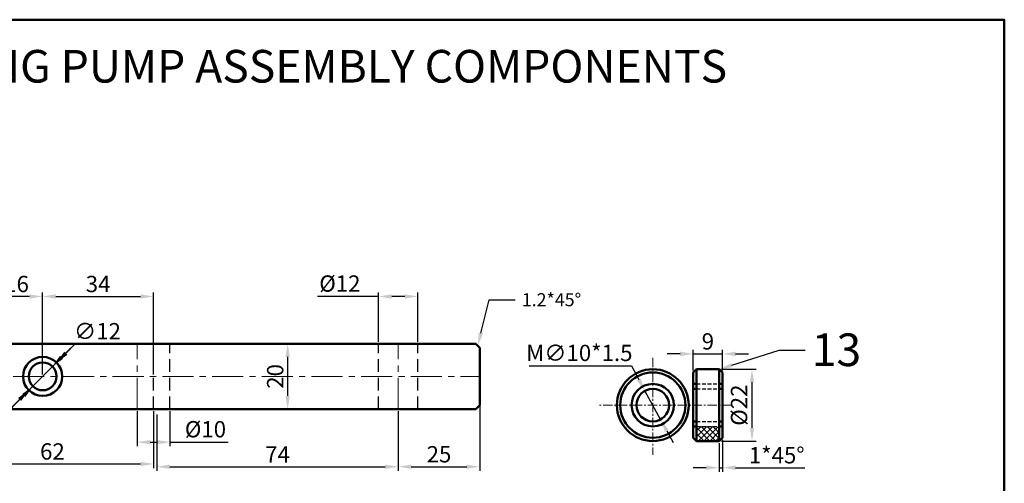
# Model space of a CAD drawing. Units: millimetres. Extents: x 24 to 508, y -182 to 223.
# Tile 6 of 6: x 207 to 508, y 81 to 223. Entities that reach past the tile are written whole.
import ezdxf
from ezdxf import colors
from ezdxf.entities.mleader import LeaderData, LeaderLine
from ezdxf.math import Vec2, Vec3

# ---------------------------------------------------------------- set-up
doc = ezdxf.new("R2010")
doc.units = ezdxf.units.MM
doc.header["$LTSCALE"] = 0.3
doc.linetypes.add('CENTER', pattern=[50.8, 31.75, -6.35, 6.35, -6.35])
doc.linetypes.add('DASHED', pattern=[19.05, 12.7, -6.35])
for name, color, linetype, lineweight in [('M-CNTR', 1, 'CENTER', 18), ('M-DIMS', 2, 'Continuous', 25), ('M-HATC', 8, 'Continuous', 18), ('M-HIDN', 4, 'DASHED', 25), ('M-OUTL', 7, 'Continuous', 50), ('M-TEXT', 7, 'Continuous', 25)]:
    doc.layers.add(name, color=color, linetype=linetype, lineweight=lineweight)
doc.styles.get("Standard").update_dxf_attribs({"font": 'arial.ttf'})
doc.dimstyles.new('ISO-25', dxfattribs={"dimtxt": 5, "dimasz": 4, "dimexe": 1.25, "dimexo": 0.625, "dimtad": 1, "dimtoh": 1, "dimdec": 0, "dimtxsty": 'Standard', "dimcen": 2.5, "dimadec": 0, "dimazin": 0, "dimtfac": 1, "dimtdec": 0, "dimtmove": 0, "dimatfit": 3, "dimfxl": 1, "dimarcsym": 0})

# ---------------------------------------------------------------- blocks, each defined once
blk = doc.blocks.new('*D8')
at = {"layer": 'Defpoints', "color": 0, "ltscale": 0.3, "transparency": 16777216}
for p in [(197.61, 137.94), (197.61, 113.44), (213.61, 113.44)]:
    blk.add_point(p, dxfattribs=at)
at = {"layer": 'M-DIMS', "color": 0, "lineweight": -2, "ltscale": 0.3, "transparency": 16777216}
for p, q in [((197.61, 114.07), (197.61, 139.19)), ((213.61, 114.07), (213.61, 139.19)), ((209.61, 137.94), (201.61, 137.94))]:
    blk.add_line(p, q, dxfattribs=at)
at = {"layer": 'M-DIMS', "color": 0, "ltscale": 0.3, "transparency": 16777216}
for points in [[(201.61, 138.6), (201.61, 137.27), (197.61, 137.94)], [(209.61, 138.6), (209.61, 137.27), (213.61, 137.94)]]:
    blk.add_solid(points, dxfattribs=at)
at = {"layer": 'M-DIMS', "color": 0, "ltscale": 0.3, "transparency": 16777216, "insert": (205.61, 141.11), "char_height": 5, "attachment_point": 5}
blk.add_mtext('16', dxfattribs=at)
blk = doc.blocks.new('*D9')
at = {"layer": 'Defpoints', "color": 0, "ltscale": 0.3, "transparency": 16777216}
for p in [(247.61, 137.94), (213.61, 113.44), (247.61, 113.44)]:
    blk.add_point(p, dxfattribs=at)
at = {"layer": 'M-DIMS', "color": 0, "lineweight": -2, "ltscale": 0.3, "transparency": 16777216}
for p, q in [((213.61, 114.07), (213.61, 139.19)), ((247.61, 114.07), (247.61, 139.19)), ((217.61, 137.94), (243.61, 137.94))]:
    blk.add_line(p, q, dxfattribs=at)
at = {"layer": 'M-DIMS', "color": 0, "ltscale": 0.3, "transparency": 16777216}
for points in [[(217.61, 138.6), (217.61, 137.27), (213.61, 137.94)], [(243.61, 138.6), (243.61, 137.27), (247.61, 137.94)]]:
    blk.add_solid(points, dxfattribs=at)
at = {"layer": 'M-DIMS', "color": 0, "ltscale": 0.3, "transparency": 16777216, "insert": (230.61, 141.12), "char_height": 5, "attachment_point": 5}
blk.add_mtext('34', dxfattribs=at)
blk = doc.blocks.new('*D10')
at = {"layer": 'Defpoints', "color": 0, "ltscale": 0.3, "transparency": 16777216}
for p in [(242.61, 103.44), (252.61, 103.44), (252.61, 93.29)]:
    blk.add_point(p, dxfattribs=at)
at = {"layer": 'M-DIMS', "color": 0, "lineweight": -2, "ltscale": 0.3, "transparency": 16777216}
for p, q in [((242.61, 102.82), (242.61, 92.04)), ((252.61, 102.82), (252.61, 92.04)), ((246.61, 93.29), (248.61, 93.29)), ((252.61, 93.29), (270.44, 93.29))]:
    blk.add_line(p, q, dxfattribs=at)
at = {"layer": 'M-DIMS', "color": 0, "ltscale": 0.3, "transparency": 16777216}
for points in [[(246.61, 93.96), (246.61, 92.63), (242.61, 93.29)], [(248.61, 93.96), (248.61, 92.63), (252.61, 93.29)]]:
    blk.add_solid(points, dxfattribs=at)
at = {"layer": 'M-DIMS', "color": 0, "ltscale": 0.3, "transparency": 16777216, "insert": (263.52, 96.61), "char_height": 5, "attachment_point": 5}
blk.add_mtext('%%C10', dxfattribs=at)
blk = doc.blocks.new('*D11')
at = {"layer": 'Defpoints', "color": 0, "ltscale": 0.3, "transparency": 16777216}
for p in [(290.14, 123.44), (288.72, 103.44), (290.14, 103.44)]:
    blk.add_point(p, dxfattribs=at)
at = {"layer": 'M-DIMS', "color": 0, "lineweight": -2, "ltscale": 0.3, "transparency": 16777216}
for p, q in [((289.51, 123.44), (287.47, 123.44)), ((288.72, 119.44), (288.72, 107.44)), ((289.51, 103.44), (287.47, 103.44))]:
    blk.add_line(p, q, dxfattribs=at)
at = {"layer": 'M-DIMS', "color": 0, "ltscale": 0.3, "transparency": 16777216}
for points in [[(288.05, 119.44), (289.39, 119.44), (288.72, 123.44)], [(288.05, 107.44), (289.39, 107.44), (288.72, 103.44)]]:
    blk.add_solid(points, dxfattribs=at)
at = {"layer": 'M-DIMS', "color": 0, "ltscale": 0.3, "transparency": 16777216, "insert": (285.54, 113.44), "char_height": 5, "attachment_point": 5, "rotation": 90}
blk.add_mtext('20', dxfattribs=at)
blk = doc.blocks.new('*D12')
at = {"layer": 'Defpoints', "color": 0, "ltscale": 0.3, "transparency": 16777216}
for p in [(347.61, 113.44), (322.61, 103.44), (347.61, 85.77)]:
    blk.add_point(p, dxfattribs=at)
at = {"layer": 'M-DIMS', "color": 0, "lineweight": -2, "ltscale": 0.3, "transparency": 16777216}
for p, q in [((347.61, 112.82), (347.61, 84.52)), ((322.61, 102.82), (322.61, 84.52)), ((326.61, 85.77), (343.61, 85.77))]:
    blk.add_line(p, q, dxfattribs=at)
at = {"layer": 'M-DIMS', "color": 0, "ltscale": 0.3, "transparency": 16777216}
for points in [[(326.61, 86.43), (326.61, 85.1), (322.61, 85.77)], [(343.61, 86.43), (343.61, 85.1), (347.61, 85.77)]]:
    blk.add_solid(points, dxfattribs=at)
at = {"layer": 'M-DIMS', "color": 0, "ltscale": 0.3, "transparency": 16777216, "insert": (335.11, 88.94), "char_height": 5, "attachment_point": 5}
blk.add_mtext('25', dxfattribs=at)
blk = doc.blocks.new('*D13')
at = {"layer": 'Defpoints', "color": 0, "ltscale": 0.3, "transparency": 16777216}
for p in [(247.61, 103.44), (185.61, 97.23), (247.61, 86.62)]:
    blk.add_point(p, dxfattribs=at)
at = {"layer": 'M-DIMS', "color": 0, "lineweight": -2, "ltscale": 0.3, "transparency": 16777216}
for p, q in [((247.61, 102.82), (247.61, 85.37)), ((185.61, 96.6), (185.61, 85.37)), ((189.61, 86.62), (243.61, 86.62))]:
    blk.add_line(p, q, dxfattribs=at)
at = {"layer": 'M-DIMS', "color": 0, "ltscale": 0.3, "transparency": 16777216}
for points in [[(189.61, 87.28), (189.61, 85.95), (185.61, 86.62)], [(243.61, 87.28), (243.61, 85.95), (247.61, 86.62)]]:
    blk.add_solid(points, dxfattribs=at)
at = {"layer": 'M-DIMS', "color": 0, "ltscale": 0.3, "transparency": 16777216, "insert": (216.61, 89.8), "char_height": 5, "attachment_point": 5}
blk.add_mtext('62', dxfattribs=at)
blk = doc.blocks.new('*D14')
at = {"layer": 'Defpoints', "color": 0, "ltscale": 0.3, "transparency": 16777216}
for p in [(322.61, 103.44), (248.61, 102.44), (322.61, 85.77)]:
    blk.add_point(p, dxfattribs=at)
at = {"layer": 'M-DIMS', "color": 0, "lineweight": -2, "ltscale": 0.3, "transparency": 16777216}
for p, q in [((322.61, 102.82), (322.61, 84.52)), ((248.61, 101.82), (248.61, 84.52)), ((252.61, 85.77), (318.61, 85.77))]:
    blk.add_line(p, q, dxfattribs=at)
at = {"layer": 'M-DIMS', "color": 0, "ltscale": 0.3, "transparency": 16777216}
for points in [[(252.61, 86.43), (252.61, 85.1), (248.61, 85.77)], [(318.61, 86.43), (318.61, 85.1), (322.61, 85.77)]]:
    blk.add_solid(points, dxfattribs=at)
at = {"layer": 'M-DIMS', "color": 0, "ltscale": 0.3, "transparency": 16777216, "insert": (285.61, 88.89), "char_height": 5, "attachment_point": 5}
blk.add_mtext('74', dxfattribs=at)
blk = doc.blocks.new('*D15')
at = {"layer": 'Defpoints', "color": 0, "ltscale": 0.3, "transparency": 16777216}
for p in [(328.61, 137.94), (316.61, 123.44), (328.61, 123.44)]:
    blk.add_point(p, dxfattribs=at)
at = {"layer": 'M-DIMS', "color": 0, "lineweight": -2, "ltscale": 0.3, "transparency": 16777216}
for p, q in [((316.61, 124.07), (316.61, 139.19)), ((328.61, 124.07), (328.61, 139.19)), ((316.61, 137.94), (297.83, 137.94)), ((324.61, 137.94), (320.61, 137.94))]:
    blk.add_line(p, q, dxfattribs=at)
at = {"layer": 'M-DIMS', "color": 0, "ltscale": 0.3, "transparency": 16777216}
for points in [[(320.61, 138.6), (320.61, 137.27), (316.61, 137.94)], [(324.61, 138.6), (324.61, 137.27), (328.61, 137.94)]]:
    blk.add_solid(points, dxfattribs=at)
at = {"layer": 'M-DIMS', "color": 0, "ltscale": 0.3, "transparency": 16777216, "insert": (304.73, 141.25), "char_height": 5, "attachment_point": 5}
blk.add_mtext('%%C12', dxfattribs=at)
blk = doc.blocks.new('*D26')
at = {"layer": 'Defpoints', "color": 0, "ltscale": 0.3, "transparency": 16777216}
for p in [(398.26, 109.03), (403.06, 100.25)]:
    blk.add_point(p, dxfattribs=at)
at = {"layer": 'M-DIMS', "color": 0, "lineweight": -2, "ltscale": 0.3, "transparency": 16777216}
for p, q in [((362.81, 116.67), (394.09, 116.67)), ((394.09, 116.67), (396.35, 112.54)), ((403.06, 100.25), (398.26, 109.03)), ((404.97, 96.74), (406.89, 93.23))]:
    blk.add_line(p, q, dxfattribs=at)
at = {"layer": 'M-DIMS', "color": 0, "ltscale": 0.3, "transparency": 16777216}
for points in [[(396.93, 112.86), (395.76, 112.22), (398.26, 109.03)], [(405.56, 97.06), (404.39, 96.42), (403.06, 100.25)]]:
    blk.add_solid(points, dxfattribs=at)
at = {"layer": 'M-DIMS', "color": 0, "ltscale": 0.3, "transparency": 16777216, "insert": (378.14, 119.99), "char_height": 5, "attachment_point": 5}
blk.add_mtext('M∅10*1.5', dxfattribs=at)
blk = doc.blocks.new('*D27')
at = {"layer": 'Defpoints', "color": 0, "ltscale": 0.3, "transparency": 16777216}
for p in [(421.05, 115.64), (421.05, 93.64), (431.07, 93.64)]:
    blk.add_point(p, dxfattribs=at)
at = {"layer": 'M-DIMS', "color": 0, "lineweight": -2, "ltscale": 0.3, "transparency": 16777216}
for p, q in [((421.68, 115.64), (432.32, 115.64)), ((431.07, 111.64), (431.07, 97.64)), ((421.68, 93.64), (432.32, 93.64))]:
    blk.add_line(p, q, dxfattribs=at)
at = {"layer": 'M-DIMS', "color": 0, "ltscale": 0.3, "transparency": 16777216}
for points in [[(430.41, 111.64), (431.74, 111.64), (431.07, 115.64)], [(430.41, 97.64), (431.74, 97.64), (431.07, 93.64)]]:
    blk.add_solid(points, dxfattribs=at)
at = {"layer": 'M-DIMS', "color": 0, "ltscale": 0.3, "transparency": 16777216, "insert": (427.76, 104.64), "char_height": 5, "attachment_point": 5, "rotation": 90}
blk.add_mtext('%%C22', dxfattribs=at)
blk = doc.blocks.new('*D28')
at = {"layer": 'Defpoints', "color": 0, "ltscale": 0.3, "transparency": 16777216}
for p in [(422.05, 120.34), (413.05, 114.64), (422.05, 114.64)]:
    blk.add_point(p, dxfattribs=at)
at = {"layer": 'M-DIMS', "color": 0, "lineweight": -2, "ltscale": 0.3, "transparency": 16777216}
for p, q in [((413.05, 115.27), (413.05, 121.59)), ((422.05, 115.27), (422.05, 121.59)), ((409.05, 120.34), (405.05, 120.34)), ((413.05, 120.34), (422.05, 120.34)), ((426.05, 120.34), (430.05, 120.34))]:
    blk.add_line(p, q, dxfattribs=at)
at = {"layer": 'M-DIMS', "color": 0, "ltscale": 0.3, "transparency": 16777216}
for points in [[(409.05, 121.01), (409.05, 119.67), (413.05, 120.34)], [(426.05, 121.01), (426.05, 119.67), (422.05, 120.34)]]:
    blk.add_solid(points, dxfattribs=at)
at = {"layer": 'M-DIMS', "color": 0, "ltscale": 0.3, "transparency": 16777216, "insert": (417.55, 123.52), "char_height": 5, "attachment_point": 5}
blk.add_mtext('9', dxfattribs=at)
blk = doc.blocks.new('*D29')
at = {"layer": 'Defpoints', "color": 0, "ltscale": 0.3, "transparency": 16777216}
for p in [(421.05, 93.64), (422.05, 94.64), (422.05, 85.46)]:
    blk.add_point(p, dxfattribs=at)
at = {"layer": 'M-DIMS', "color": 0, "lineweight": -2, "ltscale": 0.3, "transparency": 16777216}
for p, q in [((422.05, 94.02), (422.05, 84.21)), ((421.05, 93.02), (421.05, 84.21)), ((417.05, 85.46), (413.05, 85.46)), ((421.05, 85.46), (422.05, 85.46)), ((426.05, 85.46), (447.24, 85.46))]:
    blk.add_line(p, q, dxfattribs=at)
at = {"layer": 'M-DIMS', "color": 0, "ltscale": 0.3, "transparency": 16777216}
for points in [[(417.05, 86.13), (417.05, 84.8), (421.05, 85.46)], [(426.05, 86.13), (426.05, 84.8), (422.05, 85.46)]]:
    blk.add_solid(points, dxfattribs=at)
at = {"layer": 'M-DIMS', "color": 0, "ltscale": 0.3, "transparency": 16777216, "insert": (438.65, 88.64), "char_height": 5, "attachment_point": 5}
blk.add_mtext('1*45%%D', dxfattribs=at)
blk = doc.blocks.new('*D79')
at = {"layer": 'Defpoints', "color": 0, "ltscale": 0.3, "transparency": 16777216}
for p in [(217.85, 117.68), (209.36, 109.2)]:
    blk.add_point(p, dxfattribs=at)
at = {"layer": 'M-DIMS', "color": 0, "lineweight": -2, "ltscale": 0.3, "transparency": 16777216}
for p, q in [((223.51, 123.34), (220.68, 120.51)), ((236.69, 123.34), (223.51, 123.34)), ((209.36, 109.2), (217.85, 117.68)), ((206.53, 106.37), (203.7, 103.55))]:
    blk.add_line(p, q, dxfattribs=at)
at = {"layer": 'M-DIMS', "color": 0, "ltscale": 0.3, "transparency": 16777216}
for points in [[(220.21, 120.98), (221.15, 120.04), (217.85, 117.68)], [(206.06, 106.84), (207, 105.9), (209.36, 109.2)]]:
    blk.add_solid(points, dxfattribs=at)
at = {"layer": 'M-DIMS', "color": 0, "ltscale": 0.3, "transparency": 16777216, "insert": (230.41, 126.65), "char_height": 5, "attachment_point": 5}
blk.add_mtext('∅12', dxfattribs=at)
blk = doc.blocks.new('*D80')
at = {"layer": 'Defpoints', "color": 0, "ltscale": 0.3, "transparency": 16777216}
for p in [(216.59, 116.46), (210.62, 110.42)]:
    blk.add_point(p, dxfattribs=at)
at = {"layer": 'M-DIMS', "color": 0, "lineweight": -2, "ltscale": 0.3, "transparency": 16777216}
for p, q in [((219.41, 119.31), (222.22, 122.15)), ((216.59, 116.46), (210.62, 110.42)), ((201.21, 100.9), (207.81, 107.57)), ((186, 100.9), (201.21, 100.9))]:
    blk.add_line(p, q, dxfattribs=at)
at = {"layer": 'M-DIMS', "color": 0, "ltscale": 0.3, "transparency": 16777216}
for points in [[(218.93, 119.78), (219.88, 118.84), (216.59, 116.46)], [(207.33, 108.04), (208.28, 107.11), (210.62, 110.42)]]:
    blk.add_solid(points, dxfattribs=at)
at = {"layer": 'M-DIMS', "color": 0, "ltscale": 0.3, "transparency": 16777216, "insert": (193.29, 104.22), "char_height": 5, "attachment_point": 5}
blk.add_mtext('∅8.5', dxfattribs=at)

msp = doc.modelspace()

# ---------------------------------------------------------------- hatches: boundary and pattern name
at = {"layer": 'M-HATC', "ltscale": 0.3}
h = msp.add_hatch(dxfattribs=at)
h.set_pattern_fill('ANSI37', color=256, scale=0.4)
h.set_pattern_definition([(45, (7.7601, 76.6072), (-0.8980256, 0.8980256), []), (135, (7.7601, 76.6072), (-0.8980256, -0.8980256), [])])
h.paths.add_polyline_path([(414.0501, 98.1407), (414.0501, 93.6407), (421.0501, 93.6407), (421.0501, 98.1407)])

# ---------------------------------------------------------------- linework, layer by layer
at = {"layer": 'M-CNTR'}
for p, q in [((242.6065, 103.4403), (242.6065, 123.4403)), ((322.6065, 103.4403), (322.6065, 123.4403)), ((82.668, 113.4403), (347.6065, 113.4403))]:
    msp.add_line(p, q, dxfattribs=at)
at = {"layer": 'M-CNTR', "ltscale": 0.3}
for p, q in [((400.6605, 119.1069), (400.6605, 89.3694)), ((424.8527, 104.6407), (384.1108, 104.6407))]:
    msp.add_line(p, q, dxfattribs=at)
at = {"layer": 'M-HIDN'}
for p, q in [((247.6065, 103.4403), (247.6065, 123.4403)), ((252.6065, 103.4403), (252.6065, 123.4403)), ((316.6065, 103.4403), (316.6065, 123.4403)), ((328.6065, 103.4403), (328.6065, 123.4403))]:
    msp.add_line(p, q, dxfattribs=at)
at = {"layer": 'M-HIDN', "ltscale": 0.3}
for p, q in [((414.0501, 111.1407), (421.0501, 111.1407)), ((414.0501, 109.6407), (421.0501, 109.6407)), ((414.0501, 99.6407), (421.0501, 99.6407)), ((414.0501, 98.1407), (421.0501, 98.1407))]:
    msp.add_line(p, q, dxfattribs=at)
at = {"layer": 'M-OUTL'}
for p, q in [((346.4065, 123.4403), (199.6065, 123.4403)), ((346.4065, 123.4403), (347.6065, 122.2403)), ((347.6065, 104.6403), (347.6065, 122.2403)), ((346.4065, 103.4403), (199.6065, 103.4403)), ((347.6065, 104.6403), (346.4065, 103.4403))]:
    msp.add_line(p, q, dxfattribs=at)
at = {"layer": 'M-OUTL', "ltscale": 0.3}
for p, q in [((413.0501, 114.6407), (414.0501, 115.6407)), ((414.0501, 115.6407), (421.0501, 115.6407)), ((414.0501, 93.6407), (414.0501, 115.6407)), ((421.0501, 115.6407), (421.0501, 93.6407)), ((422.0501, 114.6407), (421.0501, 115.6407)), ((413.0501, 94.6407), (413.0501, 114.6407)), ((422.0501, 114.6407), (422.0501, 94.6407)), ((414.0501, 111.1407), (413.0501, 111.1407)), ((414.0501, 109.6407), (413.0501, 109.6407)), ((421.0501, 111.1407), (422.0501, 111.1407)), ((421.0501, 109.6407), (422.0501, 109.6407)), ((414.0501, 99.6407), (413.0501, 99.6407)), ((421.0501, 99.6407), (422.0501, 99.6407)), ((414.0501, 98.1407), (413.0501, 98.1407)), ((421.0501, 98.1407), (422.0501, 98.1407)), ((413.0501, 94.6407), (414.0501, 93.6407)), ((421.0501, 93.6407), (414.0501, 93.6407)), ((422.0501, 94.6407), (421.0501, 93.6407))]:
    msp.add_line(p, q, dxfattribs=at)
msp.add_lwpolyline([(23.7253, 222.7463), (508.4225, 222.7463), (508.4225, -181.5799), (23.7253, -181.5799)], close=True, dxfattribs=at)
at = {"layer": 'M-OUTL'}
for radius in [6, 4.25]:
    msp.add_circle((213.6065, 113.4403), radius, dxfattribs=at)
at = {"layer": 'M-OUTL', "ltscale": 0.3}
for radius in [11, 10, 6.5, 5]:
    msp.add_circle((400.6605, 104.6407), radius, dxfattribs=at)

# ---------------------------------------------------------------- texts
at = {"layer": 'M-TEXT', "ltscale": 0.3, "insert": (130.5797, 213.4834), "char_height": 10, "attachment_point": 1}
msp.add_mtext_dynamic_manual_height_columns('OSCILLATING PUMP ASSEMBLY COMPONENTS', width=327.515557, gutter_width=12.5, heights=[0], dxfattribs=at)

# ---------------------------------------------------------------- dimensions: what is measured, and where the dimension line sits
at = {"layer": 'M-DIMS', "ltscale": 0.3}
for base, p1, p2, picture, middle in [((197.6065, 137.9361), (213.6065, 113.4403), (197.6065, 113.4403), '*D8', (205.6065, 141.114)), ((247.6065, 137.9361), (213.6065, 113.4403), (247.6065, 113.4403), '*D9', (230.6065, 141.1157)), ((422.0501, 120.339), (413.0501, 114.6407), (422.0501, 114.6407), '*D28', (417.5501, 123.5169)), ((347.6065, 85.7656), (322.6065, 103.4403), (347.6065, 113.4403), '*D12', (335.1065, 88.9435)), ((247.6065, 86.6173), (185.6065, 97.2279), (247.6065, 103.4403), '*D13', (216.6065, 89.7952)), ((322.6065, 85.7656), (248.6065, 102.4403), (322.6065, 103.4403), '*D14', (285.6065, 88.8906))]:
    dim = msp.add_linear_dim(base=base, p1=p1, p2=p2, dimstyle='ISO-25', override={"dimclrd": 0, "dimclre": 0, "dimclrt": 0}, dxfattribs=at)
    dim.commit()
    dim.dimension.update_dxf_attribs({"geometry": picture, "text_midpoint": middle})
for base, p1, p2, picture, middle in [((328.6065, 137.9361), (316.6065, 123.4403), (328.6065, 123.4403), '*D15', (304.7306, 137.9361)), ((252.6065, 93.2948), (242.6065, 103.4403), (252.6065, 103.4403), '*D10', (263.5241, 93.2948))]:
    dim = msp.add_linear_dim(base=base, p1=p1, p2=p2, text='%%C<>', dimstyle='ISO-25', override={"dimclrd": 0, "dimclre": 0, "dimclrt": 0}, dxfattribs=at)
    dim.commit()
    dim.dimension.update_dxf_attribs({"geometry": picture, "text_midpoint": middle, "dimtype": 160})
for p1, p2, override, picture, middle in [((209.3619, 109.1996), (217.8511, 117.6811), {"dimdec": 0, "dimlfac": 1, "dimrnd": 0, "dimzin": 0, "dimdsep": 46, "dimlunit": 2}, '*D79', (230.4111, 123.3353)), ((216.5948, 116.4623), (210.6182, 110.4184), {"dimdec": 1, "dimlfac": 1, "dimrnd": 0, "dimzin": 0, "dimdsep": 46, "dimlunit": 2}, '*D80', (193.2911, 100.9006))]:
    dim = msp.add_diameter_dim_2p(p1=p1, p2=p2, dimstyle='ISO-25', override=override, dxfattribs=at)
    dim.commit()
    dim.dimension.update_dxf_attribs({"geometry": picture, "text_midpoint": middle, "dimtype": 163})
dim = msp.add_linear_dim(base=(288.7205, 103.4403), p1=(290.1379, 123.4403), p2=(290.1379, 103.4403), angle=90, dimstyle='ISO-25', override={"dimclrd": 0, "dimclre": 0, "dimclrt": 0}, dxfattribs=at)
dim.commit()
dim.dimension.update_dxf_attribs({"geometry": '*D11', "text_midpoint": (285.5426, 113.4403)})
dim = msp.add_diameter_dim_2p(p1=(403.0571, 100.2525), p2=(398.2639, 109.0289), text='M<>*1.5', dimstyle='ISO-25', override={"dimclrd": 0, "dimclre": 0, "dimclrt": 0}, dxfattribs=at)
dim.commit()
dim.dimension.update_dxf_attribs({"geometry": '*D26', "text_midpoint": (378.1376, 116.6744), "dimtype": 163})
dim = msp.add_linear_dim(base=(431.0727, 93.6407), p1=(421.0501, 115.6407), p2=(421.0501, 93.6407), angle=90, text='%%C<>', dimstyle='ISO-25', override={"dimclrd": 0, "dimclre": 0, "dimclrt": 0}, dxfattribs=at)
dim.commit()
dim.dimension.update_dxf_attribs({"geometry": '*D27', "text_midpoint": (427.755, 104.6407)})
dim = msp.add_linear_dim(base=(422.0501, 85.4633), p1=(421.0501, 93.6407), p2=(422.0501, 94.6407), text='<>*45%%D', dimstyle='ISO-25', override={"dimclrd": 0, "dimclre": 0, "dimclrt": 0}, dxfattribs=at)
dim.commit()
dim.dimension.update_dxf_attribs({"geometry": '*D29', "text_midpoint": (438.6458, 88.6412)})

# ---------------------------------------------------------------- leaders
ml = msp.add_multileader_mtext('Standard', dxfattribs=at)
ml.set_content('1.2*45%%D', color=256)
ml.set_leader_properties()
ml.build(insert=Vec2(0, 0))
ctx = ml.context
ctx.base_point, ctx.plane_origin = Vec3(358.5105, 136.9088), Vec3(347.0065, 122.8403)
notes = []
notes.append((ctx, [(0, (1, 1, 0), (350.5105, 136.9088), (1, 0), 8, [(0, [(347.0065, 122.8403)], 0, [])])]))
ctx.mtext.insert, ctx.mtext.flow_direction = Vec3(360.5105, 138.9429), 5
ml = msp.add_multileader_mtext('Standard', dxfattribs=at)
ml.set_content('13', color=256)
ml.set_leader_properties()
ml.build(insert=Vec2(0, 0))
ctx = ml.context
ctx.base_point, ctx.char_height, ctx.plane_origin = Vec3(447.3998, 121.5203), 10, Vec3(421.0501, 115.6407)
notes.append((ctx, [(0, (1, 1, 0), (439.3998, 121.5203), (1, 0), 8, [(0, [(421.0501, 115.6407)], 0, [])])]))
ctx.mtext.insert, ctx.mtext.flow_direction = Vec3(449.3998, 126.609), 5
for ctx, leaders in notes:
    for number, flags, end, landing, length, lines in leaders:
        leader = LeaderData()
        leader.index, (leader.has_last_leader_line, leader.has_dogleg_vector, leader.attachment_direction) = number, flags
        leader.last_leader_point, leader.dogleg_vector, leader.dogleg_length = Vec3(end), Vec3(landing), length
        for number, points, colour, breaks in lines:
            line = LeaderLine()
            line.index, line.vertices, line.color, line.breaks = number, Vec3.list(points), colors.encode_raw_color(colour), breaks
            leader.lines.append(line)
        ctx.leaders.append(leader)

doc.saveas('drawing.dxf')
